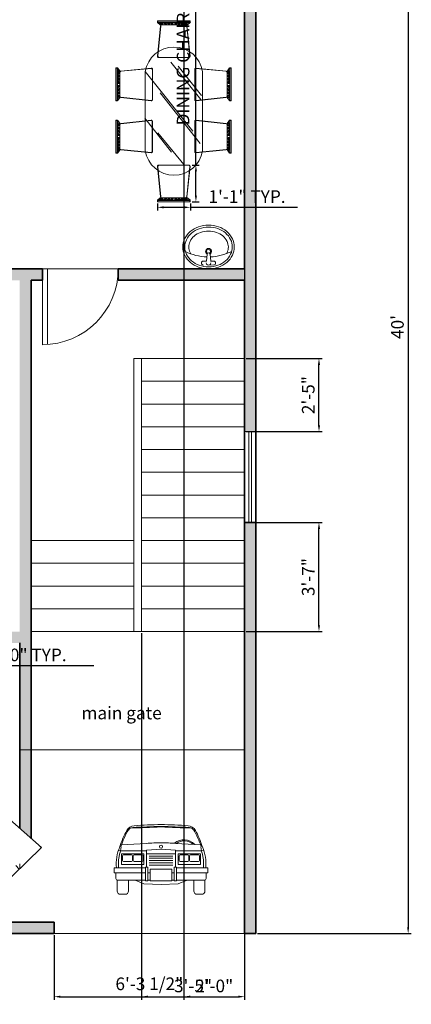
# Model space of a CAD drawing. Units: inches. Extents: x 2576 to 2974, y 2059 to 2656.
# Tile 2 of 4: x 2819 to 2974, y 2059 to 2448. Entities that reach past the tile are written whole.
import ezdxf

# ---------------------------------------------------------------- set-up
doc = ezdxf.new("R2010")
doc.units = ezdxf.units.IN
for name, color, linetype, lineweight in [('A-ANNO-DIMS', 101, 'Continuous', 18), ('A-ANNO-TEXT', 101, 'Continuous', 18), ('A-FLOR', 143, 'Continuous', 18), ('A-FLOR-FIXT', 195, 'Continuous', 18), ('A-FLOR-STRS', 143, 'Continuous', 18), ('A-WALL-PATT', 233, 'Continuous', 13), ('C-ENTG', 195, 'Continuous', 15), ('doors', 235, 'Continuous', 18), ('Furniture', 195, 'Continuous', 15), ('L-PLNT', 143, 'Continuous', 18), ('L-PLNT-PATT', 85, 'Continuous', 13), ('wall', 143, 'Continuous', 35), ('windows', 85, 'Continuous', 18)]:
    doc.layers.add(name, color=color, linetype=linetype, lineweight=lineweight)
doc.styles.get("Standard").update_dxf_attribs({"font": 'txt', "height": 5})
doc.dimstyles.new('ISO-25', dxfattribs={"dimtxt": 5, "dimasz": 2.5, "dimexe": 1.25, "dimexo": 0.625, "dimtad": 1, "dimlunit": 3, "dimtxsty": 'Standard', "dimcen": 2.5, "dimadec": 0, "dimazin": 0, "dimtfac": 1, "dimtmove": 0, "dimatfit": 3, "dimfxl": 1, "dimarcsym": 0})

# ---------------------------------------------------------------- blocks, each defined once
blk = doc.blocks.new('*D3')
at = {"layer": 'A-ANNO-DIMS', "color": 0, "lineweight": -2, "transparency": 16777216}
for p, q in [((2913.18, 2566.88), (2974.08, 2566.88)), ((2972.83, 2564.38), (2972.83, 2089.38)), ((2913.18, 2086.88), (2974.08, 2086.88))]:
    blk.add_line(p, q, dxfattribs=at)
at = {"layer": 'A-ANNO-DIMS', "color": 0, "transparency": 16777216}
for points in [[(2972.41, 2564.38), (2973.24, 2564.38), (2972.83, 2566.88)], [(2972.41, 2089.38), (2973.24, 2089.38), (2972.83, 2086.88)]]:
    blk.add_solid(points, dxfattribs=at)
at = {"layer": 'Defpoints', "color": 0, "transparency": 16777216}
for p in [(2912.56, 2566.88), (2912.56, 2086.88), (2972.83, 2086.88)]:
    blk.add_point(p, dxfattribs=at)
at = {"layer": 'A-ANNO-DIMS', "color": 0, "transparency": 16777216, "insert": (2969.23, 2326.88), "char_height": 5, "attachment_point": 5, "rotation": 90}
blk.add_mtext("40'", dxfattribs=at)
blk = doc.blocks.new('WINDOW-36IN')
for p, q in [((0, 36), (0, 0)), ((4.5, 36), (0, 36)), ((1.75, 36), (1.75, 0)), ((2.75, 36), (2.75, 0)), ((4.5, 0), (4.5, 36)), ((0, 0), (4.5, 0))]:
    blk.add_line(p, q)
blk = doc.blocks.new('CHAIR-DINING')
for p, q in [((1.24, 2.03, -2.51), (0.08, 14.01, -2.51)), ((1.35, 1.99, -2.51), (0.19, 13.97, -2.51)), ((0.52, 14.49, -2.51), (12.46, 14.5, -2.51)), ((0.63, 14.45, -2.51), (12.57, 14.46, -2.51)), ((12.89, 14.02, -2.51), (11.59, 2.03, -2.51)), ((13.01, 13.97, -2.51), (11.7, 1.99, -2.51)), ((0, 0.66, -2.51), (1.1, 1.54, -2.51)), ((12.87, 0.63, -2.51), (0, 0.61, -2.51)), ((0, 0.61, -2.51), (0, 0.04, -2.51)), ((0, 0.04, -2.51), (12.87, 0.05, -2.51)), ((0.11, 0.62, -2.51), (1.21, 1.5, -2.51)), ((12.98, 0.58, -2.51), (0.11, 0.57, -2.51)), ((0.11, 0.57, -2.51), (0.11, 0, -2.51)), ((0.11, 0, -2.51), (12.99, 0.01, -2.51)), ((2.03, 1.5, -2.51), (1.06, 0.79, -2.51)), ((1.06, 0.79, -2.51), (2.12, 0.75, -2.51)), ((1.1, 1.54, -2.51), (2.03, 1.5, -2.51)), ((2.14, 1.46, -2.51), (1.17, 0.75, -2.51)), ((1.17, 0.75, -2.51), (2.23, 0.71, -2.51)), ((1.21, 1.5, -2.51), (2.14, 1.46, -2.51)), ((11.15, 1.64, -2.51), (1.68, 1.63, -2.51)), ((11.27, 1.6, -2.51), (1.79, 1.59, -2.51)), ((2.12, 0.75, -2.51), (2.07, 1.37, -2.51)), ((2.23, 0.71, -2.51), (2.18, 1.32, -2.51)), ((2.38, 0.7, -2.51), (3.04, 1.37, -2.51)), ((2.49, 0.66, -2.51), (3.15, 1.32, -2.51)), ((3.39, 1.37, -2.51), (2.73, 0.75, -2.51)), ((2.73, 0.75, -2.51), (3, 0.75, -2.51)), ((3.51, 1.32, -2.51), (2.85, 0.71, -2.51)), ((2.85, 0.71, -2.51), (3.11, 0.71, -2.51)), ((3, 0.75, -2.51), (3.31, 1.01, -2.51)), ((3.04, 1.37, -2.51), (3.39, 1.37, -2.51)), ((3.11, 0.71, -2.51), (3.42, 0.97, -2.51)), ((3.15, 1.32, -2.51), (3.51, 1.32, -2.51)), ((3.31, 1.01, -2.51), (3.39, 0.93, -2.51)), ((3.39, 0.93, -2.51), (3.44, 1.32, -2.51)), ((3.42, 0.97, -2.51), (3.51, 0.88, -2.51)), ((3.51, 0.88, -2.51), (3.55, 1.28, -2.51)), ((3.7, 0.71, -2.51), (4.36, 1.37, -2.51)), ((3.82, 0.66, -2.51), (4.48, 1.33, -2.51)), ((4.72, 1.37, -2.51), (4.05, 0.75, -2.51)), ((4.05, 0.75, -2.51), (4.32, 0.75, -2.51)), ((4.83, 1.33, -2.51), (4.17, 0.71, -2.51)), ((4.17, 0.71, -2.51), (4.43, 0.71, -2.51)), ((4.32, 0.75, -2.51), (4.63, 1.02, -2.51)), ((4.36, 1.37, -2.51), (4.72, 1.37, -2.51)), ((4.43, 0.71, -2.51), (4.74, 0.97, -2.51)), ((4.48, 1.33, -2.51), (4.83, 1.33, -2.51)), ((4.63, 1.02, -2.51), (4.72, 0.93, -2.51)), ((4.72, 0.93, -2.51), (4.76, 1.32, -2.51)), ((4.74, 0.97, -2.51), (4.83, 0.89, -2.51)), ((4.83, 0.89, -2.51), (4.87, 1.28, -2.51)), ((5.02, 0.71, -2.51), (5.69, 1.37, -2.51)), ((5.14, 0.67, -2.51), (5.8, 1.33, -2.51)), ((6.04, 1.37, -2.51), (5.38, 0.75, -2.51)), ((5.38, 0.75, -2.51), (5.64, 0.75, -2.51)), ((6.15, 1.33, -2.51), (5.49, 0.71, -2.51)), ((5.49, 0.71, -2.51), (5.76, 0.71, -2.51)), ((5.64, 0.75, -2.51), (5.95, 1.02, -2.51)), ((5.69, 1.37, -2.51), (6.04, 1.37, -2.51)), ((5.76, 0.71, -2.51), (6.06, 0.97, -2.51)), ((5.8, 1.33, -2.51), (6.15, 1.33, -2.51)), ((5.95, 1.02, -2.51), (6.04, 0.93, -2.51)), ((6.04, 0.93, -2.51), (6.08, 1.32, -2.51)), ((6.06, 0.97, -2.51), (6.15, 0.89, -2.51)), ((6.15, 0.89, -2.51), (6.2, 1.28, -2.51)), ((6.92, 0.93, -2.51), (6.88, 1.33, -2.51)), ((7.27, 1.37, -2.51), (6.92, 1.37, -2.51)), ((6.92, 1.37, -2.51), (7.58, 0.75, -2.51)), ((7.01, 1.02, -2.51), (6.92, 0.93, -2.51)), ((7.03, 0.89, -2.51), (6.99, 1.28, -2.51)), ((7.32, 0.75, -2.51), (7.01, 1.02, -2.51)), ((7.39, 1.33, -2.51), (7.03, 1.33, -2.51)), ((7.03, 1.33, -2.51), (7.69, 0.71, -2.51)), ((7.12, 0.98, -2.51), (7.03, 0.89, -2.51)), ((7.43, 0.71, -2.51), (7.12, 0.98, -2.51)), ((7.93, 0.71, -2.51), (7.27, 1.37, -2.51)), ((7.58, 0.75, -2.51), (7.32, 0.75, -2.51)), ((8.05, 0.67, -2.51), (7.39, 1.33, -2.51)), ((7.69, 0.71, -2.51), (7.43, 0.71, -2.51)), ((8.24, 0.93, -2.51), (8.2, 1.33, -2.51)), ((8.59, 1.37, -2.51), (8.24, 1.37, -2.51)), ((8.24, 1.37, -2.51), (8.9, 0.75, -2.51)), ((8.33, 1.02, -2.51), (8.24, 0.93, -2.51)), ((8.36, 0.89, -2.51), (8.31, 1.28, -2.51)), ((8.64, 0.75, -2.51), (8.33, 1.02, -2.51)), ((8.71, 1.33, -2.51), (8.36, 1.33, -2.51)), ((8.36, 1.33, -2.51), (9.02, 0.71, -2.51)), ((8.44, 0.98, -2.51), (8.36, 0.89, -2.51)), ((8.75, 0.71, -2.51), (8.44, 0.98, -2.51)), ((9.26, 0.71, -2.51), (8.59, 1.37, -2.51)), ((8.9, 0.75, -2.51), (8.64, 0.75, -2.51)), ((9.37, 0.67, -2.51), (8.71, 1.33, -2.51)), ((9.02, 0.71, -2.51), (8.75, 0.71, -2.51)), ((9.56, 0.93, -2.51), (9.52, 1.33, -2.51)), ((9.92, 1.37, -2.51), (9.56, 1.37, -2.51)), ((9.56, 1.37, -2.51), (10.23, 0.76, -2.51)), ((9.65, 1.02, -2.51), (9.56, 0.93, -2.51)), ((9.68, 0.89, -2.51), (9.63, 1.29, -2.51)), ((9.96, 0.76, -2.51), (9.65, 1.02, -2.51)), ((10.03, 1.33, -2.51), (9.68, 1.33, -2.51)), ((9.68, 1.33, -2.51), (10.34, 0.71, -2.51)), ((9.77, 0.98, -2.51), (9.68, 0.89, -2.51)), ((10.08, 0.71, -2.51), (9.77, 0.98, -2.51)), ((10.58, 0.71, -2.51), (9.92, 1.37, -2.51)), ((10.23, 0.76, -2.51), (9.96, 0.76, -2.51)), ((10.69, 0.67, -2.51), (10.03, 1.33, -2.51)), ((10.34, 0.71, -2.51), (10.08, 0.71, -2.51)), ((10.84, 0.76, -2.51), (10.89, 1.37, -2.51)), ((11.9, 0.8, -2.51), (10.84, 0.76, -2.51)), ((11.86, 1.55, -2.51), (10.93, 1.51, -2.51)), ((10.93, 1.51, -2.51), (11.9, 0.8, -2.51)), ((10.96, 0.71, -2.51), (11, 1.33, -2.51)), ((12.01, 0.76, -2.51), (10.96, 0.71, -2.51)), ((11.97, 1.51, -2.51), (11.04, 1.46, -2.51)), ((11.04, 1.46, -2.51), (12.01, 0.76, -2.51)), ((12.96, 0.67, -2.51), (11.86, 1.55, -2.51)), ((13.07, 0.63, -2.51), (11.97, 1.51, -2.51)), ((12.87, 0.05, -2.51), (12.87, 0.63, -2.51)), ((12.99, 0.01, -2.51), (12.98, 0.58, -2.51))]:
    blk.add_line(p, q)
for centre, start, end in [((0.52, 14.05, -2.51), 90.0502, 185.5303), ((0.63, 14.01, -2.51), 90.0502, 185.5303), ((12.46, 14.06, -2.51), 353.7931, 90.0502), ((12.57, 14.02, -2.51), 353.7931, 90.0502), ((1.68, 2.07, -2.51), 185.5303, 270.0502), ((1.79, 2.03, -2.51), 185.5303, 270.0502), ((11.15, 2.08, -2.51), 270.0502, 353.7931), ((11.27, 2.04, -2.51), 270.0502, 353.7931)]:
    blk.add_arc(centre, 0.441, start, end)
blk = doc.blocks.new('*D11')
at = {"layer": 'A-ANNO-DIMS', "color": 0, "lineweight": -2, "transparency": 16777216}
for p, q in [((2688.06, 2201.25), (2688.06, 2191.63)), ((2748.06, 2201.25), (2748.06, 2191.63)), ((2690.56, 2192.88), (2745.56, 2192.88)), ((2748.06, 2192.88), (2848.47, 2192.88))]:
    blk.add_line(p, q, dxfattribs=at)
at = {"layer": 'A-ANNO-DIMS', "color": 0, "transparency": 16777216}
for points in [[(2690.56, 2193.29), (2690.56, 2192.46), (2688.06, 2192.88)], [(2745.56, 2193.29), (2745.56, 2192.46), (2748.06, 2192.88)]]:
    blk.add_solid(points, dxfattribs=at)
at = {"layer": 'Defpoints', "color": 0, "transparency": 16777216}
for p in [(2688.06, 2201.88), (2748.06, 2201.88), (2748.06, 2192.88)]:
    blk.add_point(p, dxfattribs=at)
at = {"layer": 'A-ANNO-DIMS', "color": 0, "transparency": 16777216, "insert": (2799.51, 2196.48), "char_height": 5, "attachment_point": 5}
blk.add_mtext('PAIRED DOOR 5\'-0" TYP.', dxfattribs=at)
blk = doc.blocks.new('*D15')
at = {"layer": 'A-ANNO-DIMS', "color": 0, "lineweight": -2, "transparency": 16777216}
for p, q in [((2888.82, 2390.91), (2888.82, 2508.23)), ((2887.27, 2390.91), (2890.07, 2390.91)), ((2888.82, 2378.9), (2888.82, 2388.41)), ((2887.27, 2376.4), (2890.07, 2376.4))]:
    blk.add_line(p, q, dxfattribs=at)
at = {"layer": 'A-ANNO-DIMS', "color": 0, "transparency": 16777216}
for points in [[(2888.4, 2388.41), (2889.23, 2388.41), (2888.82, 2390.91)], [(2888.4, 2378.9), (2889.23, 2378.9), (2888.82, 2376.4)]]:
    blk.add_solid(points, dxfattribs=at)
at = {"layer": 'Defpoints', "color": 0, "transparency": 16777216}
for p in [(2886.64, 2390.91), (2888.82, 2390.91), (2886.64, 2376.4)]:
    blk.add_point(p, dxfattribs=at)
at = {"layer": 'A-ANNO-DIMS', "color": 0, "transparency": 16777216, "insert": (2884.38, 2450.82), "char_height": 5, "attachment_point": 5, "rotation": 90}
blk.add_mtext('DINING CHAIR 1\'-2 1/2" TYP.', dxfattribs=at)
blk = doc.blocks.new('*D16')
at = {"layer": 'A-ANNO-DIMS', "color": 0, "lineweight": -2, "transparency": 16777216}
for p, q in [((2873.57, 2375.78), (2873.57, 2372.98)), ((2876.07, 2374.23), (2884.14, 2374.23)), ((2886.64, 2375.78), (2886.64, 2372.98)), ((2886.64, 2374.23), (2928.96, 2374.23))]:
    blk.add_line(p, q, dxfattribs=at)
at = {"layer": 'A-ANNO-DIMS', "color": 0, "transparency": 16777216}
for points in [[(2876.07, 2374.64), (2876.07, 2373.81), (2873.57, 2374.23)], [(2884.14, 2374.64), (2884.14, 2373.81), (2886.64, 2374.23)]]:
    blk.add_solid(points, dxfattribs=at)
at = {"layer": 'Defpoints', "color": 0, "transparency": 16777216}
for p in [(2873.57, 2376.4), (2886.64, 2376.4), (2886.64, 2374.23)]:
    blk.add_point(p, dxfattribs=at)
at = {"layer": 'A-ANNO-DIMS', "color": 0, "transparency": 16777216, "insert": (2909.05, 2377.83), "char_height": 5, "attachment_point": 5}
blk.add_mtext('1\'-1" TYP.', dxfattribs=at)
blk = doc.blocks.new('*D19')
at = {"layer": 'A-ANNO-DIMS', "color": 0, "lineweight": -2, "transparency": 16777216}
for p, q in [((2832.71, 2086.25), (2832.71, 2060.65)), ((2908.06, 2086.25), (2908.06, 2060.65)), ((2835.21, 2061.9), (2905.56, 2061.9))]:
    blk.add_line(p, q, dxfattribs=at)
at = {"layer": 'A-ANNO-DIMS', "color": 0, "transparency": 16777216}
for points in [[(2835.21, 2062.32), (2835.21, 2061.48), (2832.71, 2061.9)], [(2905.56, 2062.32), (2905.56, 2061.48), (2908.06, 2061.9)]]:
    blk.add_solid(points, dxfattribs=at)
at = {"layer": 'Defpoints', "color": 0, "transparency": 16777216}
for p in [(2832.71, 2086.88), (2908.06, 2086.88), (2908.06, 2061.9)]:
    blk.add_point(p, dxfattribs=at)
at = {"layer": 'A-ANNO-DIMS', "color": 0, "transparency": 16777216, "insert": (2870.38, 2066.34), "char_height": 5, "attachment_point": 5}
blk.add_mtext('6\'-3 1/2"', dxfattribs=at)
blk = doc.blocks.new('*D20')
at = {"layer": 'A-ANNO-DIMS', "color": 0, "lineweight": -2, "transparency": 16777216}
for p, q in [((2867.31, 2205.75), (2867.31, 2060.65)), ((2908.06, 2205.75), (2908.06, 2060.65)), ((2869.81, 2061.9), (2905.56, 2061.9))]:
    blk.add_line(p, q, dxfattribs=at)
at = {"layer": 'A-ANNO-DIMS', "color": 0, "transparency": 16777216}
for points in [[(2869.81, 2062.32), (2869.81, 2061.48), (2867.31, 2061.9)], [(2905.56, 2062.32), (2905.56, 2061.48), (2908.06, 2061.9)]]:
    blk.add_solid(points, dxfattribs=at)
at = {"layer": 'Defpoints', "color": 0, "transparency": 16777216}
for p in [(2867.31, 2206.38), (2908.06, 2206.38), (2908.06, 2061.9)]:
    blk.add_point(p, dxfattribs=at)
at = {"layer": 'A-ANNO-DIMS', "color": 0, "transparency": 16777216, "insert": (2887.68, 2065.5), "char_height": 5, "attachment_point": 5}
blk.add_mtext('3\'-5"', dxfattribs=at)
blk = doc.blocks.new('*D21')
at = {"layer": 'A-ANNO-DIMS', "color": 0, "lineweight": -2, "transparency": 16777216}
for p, q in [((2908.68, 2314.38), (2938.78, 2314.38)), ((2937.53, 2287.99), (2937.53, 2311.88)), ((2908.68, 2285.49), (2938.78, 2285.49))]:
    blk.add_line(p, q, dxfattribs=at)
at = {"layer": 'A-ANNO-DIMS', "color": 0, "transparency": 16777216}
for points in [[(2937.11, 2311.88), (2937.95, 2311.88), (2937.53, 2314.38)], [(2937.11, 2287.99), (2937.95, 2287.99), (2937.53, 2285.49)]]:
    blk.add_solid(points, dxfattribs=at)
at = {"layer": 'Defpoints', "color": 0, "transparency": 16777216}
for p in [(2908.06, 2314.38), (2937.53, 2314.38), (2908.06, 2285.49)]:
    blk.add_point(p, dxfattribs=at)
at = {"layer": 'A-ANNO-DIMS', "color": 0, "transparency": 16777216, "insert": (2933.93, 2299.93), "char_height": 5, "attachment_point": 5, "rotation": 90}
blk.add_mtext('2\'-5"', dxfattribs=at)
blk = doc.blocks.new('*D36')
at = {"layer": 'A-ANNO-DIMS', "color": 0, "lineweight": -2, "transparency": 16777216}
for p, q in [((2908.68, 2249.49), (2938.78, 2249.49)), ((2937.53, 2208.88), (2937.53, 2246.99)), ((2908.68, 2206.38), (2938.78, 2206.38))]:
    blk.add_line(p, q, dxfattribs=at)
at = {"layer": 'A-ANNO-DIMS', "color": 0, "transparency": 16777216}
for points in [[(2937.11, 2246.99), (2937.95, 2246.99), (2937.53, 2249.49)], [(2937.11, 2208.88), (2937.95, 2208.88), (2937.53, 2206.38)]]:
    blk.add_solid(points, dxfattribs=at)
at = {"layer": 'Defpoints', "color": 0, "transparency": 16777216}
for p in [(2908.06, 2249.49), (2937.53, 2249.49), (2908.06, 2206.38)]:
    blk.add_point(p, dxfattribs=at)
at = {"layer": 'A-ANNO-DIMS', "color": 0, "transparency": 16777216, "insert": (2933.93, 2227.93), "char_height": 5, "attachment_point": 5, "rotation": 90}
blk.add_mtext('3\'-7"', dxfattribs=at)
blk = doc.blocks.new('*D38')
at = {"layer": 'A-ANNO-DIMS', "color": 0, "lineweight": -2, "transparency": 16777216}
for p, q in [((2884.06, 2459.75), (2884.06, 2060.65)), ((2908.06, 2459.75), (2908.06, 2060.65)), ((2886.56, 2061.9), (2905.56, 2061.9))]:
    blk.add_line(p, q, dxfattribs=at)
at = {"layer": 'A-ANNO-DIMS', "color": 0, "transparency": 16777216}
for points in [[(2886.56, 2062.32), (2886.56, 2061.48), (2884.06, 2061.9)], [(2905.56, 2062.32), (2905.56, 2061.48), (2908.06, 2061.9)]]:
    blk.add_solid(points, dxfattribs=at)
at = {"layer": 'Defpoints', "color": 0, "transparency": 16777216}
for p in [(2884.06, 2460.38), (2908.06, 2460.38), (2908.06, 2061.9)]:
    blk.add_point(p, dxfattribs=at)
at = {"layer": 'A-ANNO-DIMS', "color": 0, "transparency": 16777216, "insert": (2896.06, 2065.5), "char_height": 5, "attachment_point": 5}
blk.add_mtext('2\'-0"', dxfattribs=at)

msp = doc.modelspace()

# ---------------------------------------------------------------- hatches: boundary and pattern name
at = {"layer": 'A-WALL-PATT'}
h = msp.add_hatch(color=256, dxfattribs=at)
h.dxf.hatch_style = 1
h.paths.add_polyline_path([(2726.595, 2349.876), (2706.556, 2349.876), (2706.556, 2381.376), (2702.056, 2381.376), (2702.056, 2349.876), (2617.056, 2349.876), (2617.056, 2370.876), (2612.556, 2370.876), (2612.556, 2287.457), (2617.056, 2287.457), (2617.056, 2345.376), (2726.595, 2345.376)])
h.paths.add_polyline_path([(2823.556, 2345.376), (2828.056, 2345.376), (2828.056, 2349.876), (2808.018, 2349.876), (2808.018, 2345.376), (2819.056, 2345.376), (2819.056, 2206.376), (2748.056, 2206.376), (2748.056, 2201.876), (2819.056, 2201.876), (2819.056, 2159.528), (2823.556, 2159.528)])
h.paths.add_polyline_path([(2634.556, 2206.376), (2617.056, 2206.376), (2617.056, 2239.457), (2612.556, 2239.457), (2612.556, 2086.876), (2696.755, 2086.876), (2696.755, 2091.376), (2617.056, 2091.376), (2617.056, 2201.876), (2634.556, 2201.876)])
h.paths.add_polyline_path([(2688.056, 2206.376), (2670.556, 2206.376), (2670.556, 2201.876), (2688.056, 2201.876)], flags=17)
h.paths.add_polyline_path([(2832.708, 2091.376), (2732.755, 2091.376), (2732.755, 2086.876), (2832.708, 2086.876)])
h.paths.add_polyline_path([(2823.556, 2159.528), (2819.056, 2159.528), (2819.056, 2128.522), (2823.556, 2124.554)])
h.paths.add_polyline_path([(2840.936, 2566.876), (2689.889, 2566.876), (2689.889, 2562.376), (2730.206, 2562.376), (2737.056, 2562.376), (2737.056, 2529.376), (2741.556, 2529.376), (2741.556, 2562.376), (2813.556, 2562.376), (2813.556, 2529.376), (2818.056, 2529.376), (2818.056, 2562.376), (2840.936, 2562.376)])
h.paths.add_polyline_path([(2653.889, 2566.876), (2612.556, 2566.876), (2612.556, 2509.376), (2617.056, 2509.376), (2617.056, 2562.376), (2653.889, 2562.376)])
h.paths.add_polyline_path([(2822.556, 2460.376), (2818.056, 2460.376), (2818.056, 2493.376), (2813.556, 2493.376), (2813.556, 2460.376), (2809.817, 2460.376), (2809.817, 2455.876), (2822.556, 2455.876)])
h.paths.add_polyline_path([(2912.556, 2489.593), (2908.056, 2489.593), (2908.056, 2470.164), (2908.056, 2460.376), (2852.556, 2460.376), (2852.556, 2455.876), (2908.056, 2455.876), (2908.056, 2349.876), (2858.056, 2349.876), (2858.056, 2345.376), (2908.056, 2345.376), (2908.056, 2285.493), (2912.556, 2285.493)])
h.paths.add_polyline_path([(2749.817, 2460.376), (2741.556, 2460.376), (2741.556, 2493.376), (2737.056, 2493.376), (2737.056, 2450.376), (2741.556, 2450.376), (2741.556, 2455.876), (2749.817, 2455.876)])
h.paths.add_polyline_path([(2741.556, 2420.376), (2711.556, 2420.376), (2617.056, 2420.376), (2617.056, 2473.376), (2612.556, 2473.376), (2612.556, 2394.876), (2617.056, 2394.876), (2617.056, 2415.876), (2702.056, 2415.876), (2702.056, 2411.376), (2706.556, 2411.376), (2706.556, 2415.876), (2741.556, 2415.876)])
h.paths.add_polyline_path([(2912.556, 2566.876), (2876.936, 2566.876), (2876.936, 2562.376), (2908.056, 2562.376), (2908.056, 2525.593), (2912.556, 2525.593)])
h.paths.add_polyline_path([(2741.924, 2553.087), (2815.278, 2553.087), (2815.278, 2560.74), (2741.924, 2560.74)], flags=25)
h = msp.add_hatch(color=256, dxfattribs=at)
h.dxf.hatch_style = 1
h.paths.add_polyline_path([(2912.556, 2249.493), (2908.056, 2249.493), (2908.056, 2086.876), (2912.556, 2086.876)])
at = {"layer": 'L-PLNT-PATT'}
h = msp.add_hatch(dxfattribs=at)
h.set_pattern_fill('GRASS', color=256, scale=0.48)
h.paths.add_polyline_path([(2827.63, 2120.961), (2783.902, 2159.528), (2617.056, 2159.528), (2617.056, 2091.376), (2797.373, 2091.376)])

# ---------------------------------------------------------------- linework, layer by layer
at = {"layer": 'A-FLOR'}
msp.add_line((2819.056, 2159.528), (2908.056, 2159.528), dxfattribs=at)
at = {"layer": 'A-FLOR-FIXT'}
for p, q in [((2892.952, 2352.92), (2893.237, 2355.677)), ((2894.713, 2352.926), (2894.408, 2355.681)), ((2891.762, 2352.932), (2893.001, 2352.937)), ((2895.862, 2351.411), (2893.815, 2351.286)), ((2895.857, 2352.946), (2894.618, 2352.942))]:
    msp.add_line(p, q, dxfattribs=at)
for centre, radius, start, end in [((2893.249, 2356.843), 10.257, 109.58097, 130.54225), ((2893.249, 2356.843), 9.469, 109.58097, 130.54225), ((2893.824, 2355.224), 11.974, 90.19698, 109.58097), ((2893.824, 2355.224), 11.187, 90.19698, 109.58097), ((2893.824, 2355.224), 9.612, 90.19698, 109.58097), ((2893.824, 2355.224), 11.974, 70.81298, 90.19698), ((2893.824, 2355.224), 11.187, 70.81298, 90.19698), ((2893.824, 2355.224), 9.612, 70.81298, 90.19698), ((2894.389, 2356.847), 9.469, 49.85171, 70.81298), ((2894.389, 2356.847), 10.257, 49.85171, 70.81298), ((2891.012, 2358.528), 7.396, 154.20116, 180.19698), ((2892.368, 2357.872), 8.902, 130.54225, 154.20116), ((2891.012, 2358.528), 6.608, 154.20116, 180.19698), ((2892.368, 2357.872), 8.115, 130.54225, 154.20116), ((2892.368, 2357.872), 6.54, 130.54225, 154.20116), ((2893.249, 2356.843), 7.895, 109.58097, 130.54225), ((2894.389, 2356.847), 7.895, 49.85171, 70.81298), ((2895.262, 2357.882), 6.54, 26.1928, 49.85171), ((2895.262, 2357.882), 8.115, 26.1928, 49.85171), ((2895.262, 2357.882), 8.902, 26.1928, 49.85171), ((2896.614, 2358.547), 6.608, 0.19698, 26.1928), ((2896.614, 2358.547), 7.396, 0.19698, 26.1928), ((2891.012, 2358.528), 7.396, 180.19698, 206.1928), ((2891.012, 2358.528), 6.608, 180.19698, 206.1928), ((2891.012, 2358.528), 5.033, 154.20116, 180.19698), ((2891.012, 2358.528), 5.033, 180.19698, 206.1928), ((2893.819, 2356.766), 1.181, 299.152, 241.24195), ((2893.819, 2356.766), 0.787, 296.58131, 243.81265), ((2896.614, 2358.547), 5.033, 0.19698, 26.1928), ((2896.614, 2358.547), 5.033, 334.20116, 0.19698), ((2896.614, 2358.547), 6.608, 334.20116, 0.19698), ((2896.614, 2358.547), 7.396, 334.20116, 0.19698), ((2892.364, 2359.193), 8.902, 206.1928, 229.85171), ((2893.756, 2375.089), 20.489, 243.61779, 268.23969), ((2892.364, 2359.193), 8.115, 206.1928, 229.85171), ((2892.364, 2359.193), 6.54, 206.1928, 210.89435), ((2893.823, 2355.585), 0.591, 9.39225, 171.00171), ((2893.756, 2375.089), 20.489, 272.15427, 296.77617), ((2895.258, 2359.203), 8.115, 310.54225, 334.20116), ((2895.258, 2359.203), 6.54, 329.4996, 334.20116), ((2895.258, 2359.203), 8.902, 310.54225, 334.20116), ((2893.237, 2360.228), 10.257, 229.85171, 250.81298), ((2893.237, 2360.228), 9.469, 229.85171, 250.81298), ((2893.802, 2361.85), 11.974, 250.81298, 270.19698), ((2893.802, 2361.85), 11.187, 250.81298, 270.19698), ((2891.765, 2352.165), 0.768, 90.19698, 270.19698), ((2893.812, 2352.172), 0.886, 174.08148, 6.31248), ((2893.802, 2361.85), 11.187, 270.19698, 289.58097), ((2893.802, 2361.85), 11.974, 270.19698, 289.58097), ((2895.859, 2352.179), 0.768, 270.19698, 90.19698), ((2894.377, 2360.232), 9.469, 289.58097, 310.54225), ((2894.377, 2360.232), 10.257, 289.58097, 310.54225)]:
    msp.add_arc(centre, radius, start, end, dxfattribs=at)
at = {"layer": 'A-FLOR-STRS'}
for p, q in [((2864.306, 2314.376), (2908.056, 2314.376)), ((2864.306, 2206.376), (2864.306, 2314.376)), ((2867.306, 2206.376), (2867.306, 2314.376)), ((2867.306, 2305.376), (2908.056, 2305.376)), ((2867.306, 2296.376), (2908.056, 2296.376)), ((2867.306, 2287.376), (2908.056, 2287.376)), ((2867.306, 2278.376), (2908.056, 2278.376)), ((2867.306, 2269.376), (2908.056, 2269.376)), ((2867.306, 2260.376), (2908.056, 2260.376)), ((2867.306, 2251.376), (2908.056, 2251.376)), ((2823.556, 2242.376), (2864.306, 2242.376)), ((2867.306, 2242.376), (2908.056, 2242.376)), ((2823.556, 2233.376), (2864.306, 2233.376)), ((2867.306, 2233.376), (2908.056, 2233.376)), ((2823.556, 2224.376), (2864.306, 2224.376)), ((2867.306, 2224.376), (2908.056, 2224.376)), ((2823.556, 2215.376), (2864.306, 2215.376)), ((2867.306, 2215.376), (2908.056, 2215.376)), ((2823.556, 2206.376), (2908.056, 2206.376))]:
    msp.add_line(p, q, dxfattribs=at)
at = {"layer": 'C-ENTG'}
for p, q in [((2858.917, 2119.578), (2858.165, 2119.672)), ((2858.732, 2119.588), (2869.313, 2119.588)), ((2859.218, 2121.242), (2858.823, 2118.826)), ((2869.238, 2122.558), (2859.218, 2122.032)), ((2869.313, 2119.919), (2875.015, 2120.27)), ((2869.313, 2113.092), (2869.313, 2119.919)), ((2880.717, 2119.919), (2875.015, 2120.27)), ((2880.717, 2113.092), (2880.717, 2119.919)), ((2891.299, 2119.588), (2880.717, 2119.588)), ((2880.793, 2122.558), (2890.812, 2122.032)), ((2890.812, 2121.242), (2891.208, 2118.826)), ((2891.113, 2119.578), (2891.866, 2119.672)), ((2858.739, 2118.799), (2858.165, 2116.097)), ((2858.165, 2116.097), (2858.165, 2112.913)), ((2859.404, 2114.186), (2859.404, 2118.457)), ((2859.404, 2118.457), (2868.257, 2118.457)), ((2859.797, 2117.66), (2859.797, 2115.79)), ((2863.324, 2118.048), (2860.185, 2118.048)), ((2863.712, 2117.66), (2863.712, 2115.79)), ((2863.978, 2117.66), (2863.978, 2115.79)), ((2867.505, 2118.048), (2864.366, 2118.048)), ((2867.893, 2115.79), (2867.893, 2117.66)), ((2868.257, 2118.457), (2868.257, 2114.186)), ((2869.313, 2118.457), (2875.015, 2118.457)), ((2875.015, 2117.55), (2870.322, 2117.55)), ((2875.015, 2116.657), (2870.322, 2116.657)), ((2875.015, 2115.763), (2870.322, 2115.763)), ((2880.717, 2118.457), (2875.015, 2118.457)), ((2875.015, 2117.55), (2879.709, 2117.55)), ((2875.015, 2116.657), (2879.709, 2116.657)), ((2875.015, 2115.763), (2879.709, 2115.763)), ((2890.627, 2118.457), (2881.774, 2118.457)), ((2881.774, 2118.457), (2881.774, 2114.186)), ((2882.138, 2115.79), (2882.138, 2117.66)), ((2882.526, 2118.048), (2885.664, 2118.048)), ((2886.052, 2117.66), (2886.052, 2115.79)), ((2886.319, 2117.66), (2886.319, 2115.79)), ((2886.707, 2118.048), (2889.846, 2118.048)), ((2890.233, 2117.66), (2890.233, 2115.79)), ((2890.627, 2114.186), (2890.627, 2118.457)), ((2891.292, 2118.799), (2891.866, 2116.097)), ((2891.866, 2116.097), (2891.866, 2112.913)), ((2856.477, 2112.913), (2868.856, 2112.913)), ((2856.477, 2110.854), (2856.477, 2112.913)), ((2868.257, 2114.186), (2859.404, 2114.186)), ((2860.185, 2115.402), (2863.324, 2115.402)), ((2864.366, 2115.402), (2867.505, 2115.402)), ((2868.856, 2113.092), (2868.856, 2107.749)), ((2869.771, 2113.092), (2868.856, 2113.092)), ((2869.771, 2107.749), (2869.771, 2113.092)), ((2875.015, 2114.869), (2870.322, 2114.869)), ((2875.015, 2113.975), (2870.322, 2113.975)), ((2870.687, 2107.701), (2870.687, 2112.383)), ((2870.687, 2112.383), (2875.015, 2112.383)), ((2875.015, 2114.869), (2879.709, 2114.869)), ((2875.015, 2113.975), (2879.709, 2113.975)), ((2879.344, 2112.383), (2875.015, 2112.383)), ((2879.344, 2107.701), (2879.344, 2112.383)), ((2880.259, 2113.092), (2881.175, 2113.092)), ((2880.259, 2107.749), (2880.259, 2113.092)), ((2881.175, 2113.092), (2881.175, 2107.749)), ((2893.553, 2112.913), (2881.175, 2112.913)), ((2881.774, 2114.186), (2890.627, 2114.186)), ((2885.664, 2115.402), (2882.526, 2115.402)), ((2889.846, 2115.402), (2886.707, 2115.402)), ((2893.553, 2110.854), (2893.553, 2112.913)), ((2856.477, 2110.854), (2868.856, 2110.854)), ((2857.168, 2108.615), (2857.168, 2110.864)), ((2857.645, 2103.7), (2857.645, 2108.006)), ((2857.823, 2108.006), (2868.856, 2108.006)), ((2862.072, 2108.006), (2862.072, 2103.7)), ((2868.222, 2106.575), (2864.712, 2107.977)), ((2868.856, 2107.749), (2869.771, 2107.749)), ((2869.771, 2110.854), (2870.687, 2110.854)), ((2869.771, 2108.006), (2870.687, 2108.006)), ((2875.015, 2107.701), (2870.687, 2107.701)), ((2875.015, 2107.701), (2879.344, 2107.701)), ((2879.344, 2110.854), (2880.259, 2110.854)), ((2880.259, 2108.006), (2879.344, 2108.006)), ((2881.175, 2107.749), (2880.259, 2107.749)), ((2893.553, 2110.854), (2881.175, 2110.854)), ((2892.208, 2108.006), (2881.175, 2108.006)), ((2881.808, 2106.575), (2885.318, 2107.977)), ((2887.959, 2108.006), (2887.959, 2103.7)), ((2892.385, 2103.7), (2892.385, 2108.006)), ((2892.863, 2108.615), (2892.863, 2110.864)), ((2868.222, 2106.575), (2875.015, 2106.341)), ((2881.808, 2106.575), (2875.015, 2106.341)), ((2860.779, 2102.407), (2858.938, 2102.407)), ((2889.252, 2102.407), (2891.093, 2102.407))]:
    msp.add_line(p, q, dxfattribs=at)
msp.add_circle((2875.015, 2121.277), 0.624, dxfattribs=at)
for centre, radius, start, end in [((2893.785, 2110.012), 36.859, 151.35207, 162.17305), ((2888.338, 2112.205), 30.579, 149.24853, 162.62993), ((2864.591, 2125.897), 3.62, 94.35225, 150.45231), ((2863.86, 2126.786), 2.068, 92.15835, 149.65533), ((2447.458, 13187.363), 11066.573, 272.1511059, 272.2141727), ((2447.458, 13187.593), 11066.573, 272.15597, 272.2141727), ((2876.567, 1974.298), 155.696, 90.5709, 94.51299), ((2873.464, 1974.298), 155.696, 85.48701, 89.4291), ((3302.572, 13187.593), 11066.573, 267.7858273, 267.84403), ((3302.572, 13187.363), 11066.573, 267.7858273, 267.8488941), ((2885.44, 2125.897), 3.62, 29.54769, 85.64775), ((2886.171, 2126.786), 2.068, 30.34467, 87.84165), ((2861.692, 2112.205), 30.579, 17.37007, 30.75147), ((2856.246, 2110.012), 36.859, 17.82695, 28.64793), ((2884.161, 2118.307), 5.699, 42.53927, 131.31695), ((2884.161, 2118.307), 5.224, 48.13217, 125.8531), ((2874.148, 2114.473), 16.9, 156.62619, 185.29362), ((2876.567, 2027.915), 94.926, 90.9364, 94.42783), ((2873.464, 2027.915), 94.926, 85.57217, 89.0636), ((2875.883, 2114.473), 16.9, 354.70638, 23.37381), ((2860.185, 2117.66), 0.388, 90, 180), ((2860.185, 2115.79), 0.388, 180, 270), ((2863.324, 2117.66), 0.388, 0, 90), ((2863.324, 2115.79), 0.388, 270, 0), ((2864.366, 2117.66), 0.388, 90, 180), ((2864.366, 2115.79), 0.388, 180, 270), ((2867.505, 2117.66), 0.388, 0, 90), ((2867.505, 2115.79), 0.388, 270, 0), ((2882.526, 2117.66), 0.388, 90, 180), ((2882.526, 2115.79), 0.388, 180, 270), ((2885.664, 2117.66), 0.388, 0, 90), ((2885.664, 2115.79), 0.388, 270, 0), ((2886.707, 2117.66), 0.388, 90, 180), ((2886.707, 2115.79), 0.388, 180, 270), ((2889.846, 2117.66), 0.388, 0, 90), ((2889.846, 2115.79), 0.388, 270, 0), ((2857.925, 2108.782), 0.776, 192.40742, 270), ((2892.105, 2108.782), 0.776, 270, 347.59258), ((2858.938, 2103.7), 1.293, 180, 270), ((2860.779, 2103.7), 1.293, 270, 0), ((2889.252, 2103.7), 1.293, 180, 270), ((2891.093, 2103.7), 1.293, 270, 0)]:
    msp.add_arc(centre, radius, start, end, dxfattribs=at)
at = {"layer": 'doors'}
for p, q in [((2828.056, 2319.876), (2828.056, 2349.876)), ((2828.056, 2349.876), (2858.056, 2349.876)), ((2830.056, 2319.943), (2830.056, 2349.876)), ((2832.708, 2086.876), (2908.056, 2086.876))]:
    msp.add_line(p, q, dxfattribs=at)
msp.add_arc((2828.056, 2349.876), 30, 270, 0, dxfattribs=at)
at = {"layer": 'Furniture'}
for p, q in [((2878.874, 2431.705), (2890.764, 2416.905)), ((2868.762, 2427.987), (2887.55, 2404.358)), ((2868.762, 2427.987), (2868.762, 2396.594)), ((2881.766, 2430.096), (2891.085, 2418.514)), ((2891.444, 2396.594), (2891.444, 2427.987)), ((2874.697, 2419.479), (2890.443, 2399.531)), ((2868.591, 2409.505), (2879.195, 2395.992)), ((2873.733, 2403.714), (2884.016, 2391.166))]:
    msp.add_line(p, q, dxfattribs=at)
for centre, start, end in [((2880.103, 2426.164), 9.13208, 170.86792), ((2880.103, 2398.417), 189.13208, 350.86792)]:
    msp.add_arc(centre, 11.487, start, end, dxfattribs=at)
at = {"layer": 'L-PLNT'}
for p, q in [((2783.902, 2159.528), (2827.63, 2120.961)), ((2827.63, 2120.961), (2797.373, 2091.376))]:
    msp.add_line(p, q, dxfattribs=at)
at = {"layer": 'wall'}
for p, q in [((2912.556, 2566.876), (2912.556, 2086.876)), ((2908.056, 2455.876), (2908.056, 2349.876)), ((2808.018, 2349.876), (2828.056, 2349.876)), ((2828.056, 2345.376), (2828.056, 2349.876)), ((2858.056, 2345.376), (2858.056, 2349.876)), ((2858.056, 2349.876), (2908.056, 2349.876)), ((2823.556, 2124.554), (2823.556, 2345.376)), ((2823.556, 2345.376), (2828.056, 2345.376)), ((2858.056, 2345.376), (2908.056, 2345.376)), ((2908.056, 2345.376), (2908.056, 2086.876)), ((2819.056, 2128.522), (2819.056, 2201.876)), ((2832.708, 2091.376), (2617.056, 2091.376)), ((2832.708, 2086.876), (2832.708, 2091.376)), ((2832.708, 2086.876), (2612.556, 2086.876)), ((2912.556, 2086.876), (2908.056, 2086.876))]:
    msp.add_line(p, q, dxfattribs=at)
msp.add_lwpolyline([(2912.556, 2086.876), (2908.056, 2086.876), (2908.056, 2249.493), (2912.556, 2249.493)], close=True, dxfattribs=at)

# ---------------------------------------------------------------- block references
at = {"layer": 'Furniture', "extrusion": (0, 0, -1), "zscale": -1}
for p, rotation in [((-2873.568, 2448.014), 180), ((-2902.812, 2429.395), 269.9497778456612), ((-2857.1, 2395.691), 90.00000000000163)]:
    msp.add_blockref('CHAIR-DINING', p, dxfattribs=dict(at, rotation=rotation))
at = {"layer": 'Furniture'}
for p, rotation in [((2857.115, 2429.395), 269.9497778456428), ((2902.827, 2395.691), 89.99999999999483)]:
    msp.add_blockref('CHAIR-DINING', p, dxfattribs=dict(at, rotation=rotation))
msp.add_blockref('CHAIR-DINING', (2873.568, 2376.402), dxfattribs=at)
at = {"layer": 'windows'}
msp.add_blockref('WINDOW-36IN', (2908.056, 2249.493), dxfattribs=at)

# ---------------------------------------------------------------- texts
at = {"layer": 'A-ANNO-TEXT'}
msp.add_text('main gate', height=5, dxfattribs=at).set_placement((2843.514, 2171.643))

# ---------------------------------------------------------------- dimensions: what is measured, and where the dimension line sits
at = {"layer": 'A-ANNO-DIMS'}
for base, p1, p2, override, picture, middle in [((2972.827, 2086.876), (2912.556, 2566.876), (2912.556, 2086.876), {"dimclrd": 0, "dimclre": 0, "dimclrt": 0}, '*D3', (2969.226, 2326.876)), ((2937.531, 2314.376), (2908.056, 2285.493), (2908.056, 2314.376), {"dimdec": 1, "dimlfac": 1, "dimrnd": 0, "dimzin": 1, "dimdsep": 46, "dimlunit": 4, "dimfrac": 2}, '*D21', (2933.93, 2299.934)), ((2937.531, 2249.493), (2908.056, 2206.376), (2908.056, 2249.493), {"dimdec": 1, "dimlfac": 1, "dimrnd": 0, "dimzin": 1, "dimdsep": 46, "dimlunit": 4, "dimfrac": 2}, '*D36', (2933.93, 2227.934))]:
    dim = msp.add_linear_dim(base=base, p1=p1, p2=p2, angle=90, dimstyle='ISO-25', override=override, dxfattribs=at)
    dim.commit()
    dim.dimension.update_dxf_attribs({"geometry": picture, "text_midpoint": middle})
dim = msp.add_linear_dim(base=(2888.816, 2390.906), p1=(2886.641, 2376.402), p2=(2886.641, 2390.906), angle=90, text='DINING CHAIR <> TYP.', dimstyle='ISO-25', override={"dimdec": 1, "dimlfac": 1, "dimrnd": 0, "dimzin": 1, "dimdsep": 46, "dimlunit": 4, "dimfrac": 2}, dxfattribs=at)
dim.commit()
dim.dimension.update_dxf_attribs({"geometry": '*D15', "text_midpoint": (2884.382, 2450.816)})
for base, p1, p2, picture, middle in [((2908.056, 2061.901), (2884.056, 2460.376), (2908.056, 2460.376), '*D38', (2896.056, 2065.502)), ((2908.056206, 2061.900908), (2867.306206, 2206.375908), (2908.056206, 2206.375908), '*D20', (2887.681206, 2065.502098476)), ((2908.056, 2061.901), (2832.708, 2086.876), (2908.056, 2086.876), '*D19', (2870.382, 2066.335))]:
    dim = msp.add_linear_dim(base=base, p1=p1, p2=p2, dimstyle='ISO-25', override={"dimdec": 1, "dimlfac": 1, "dimrnd": 0, "dimzin": 1, "dimdsep": 46, "dimlunit": 4, "dimfrac": 2}, dxfattribs=at)
    dim.commit()
    dim.dimension.update_dxf_attribs({"geometry": picture, "text_midpoint": middle})
for base, p1, p2, text, picture, middle in [((2886.641, 2374.226), (2873.568, 2376.402), (2886.641, 2376.402), '<> TYP.', '*D16', (2909.051, 2377.828)), ((2748.056, 2192.876), (2688.056, 2201.876), (2748.056, 2201.876), 'PAIRED DOOR <> TYP.', '*D11', (2799.515, 2196.477))]:
    dim = msp.add_linear_dim(base=base, p1=p1, p2=p2, text=text, dimstyle='ISO-25', override={"dimdec": 1, "dimlfac": 1, "dimrnd": 0, "dimzin": 1, "dimdsep": 46, "dimlunit": 4, "dimfrac": 2}, dxfattribs=at)
    dim.commit()
    dim.dimension.update_dxf_attribs({"geometry": picture, "text_midpoint": middle})

doc.saveas('drawing.dxf')
